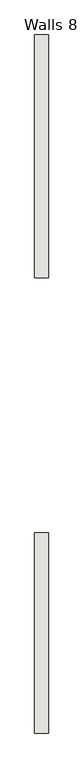
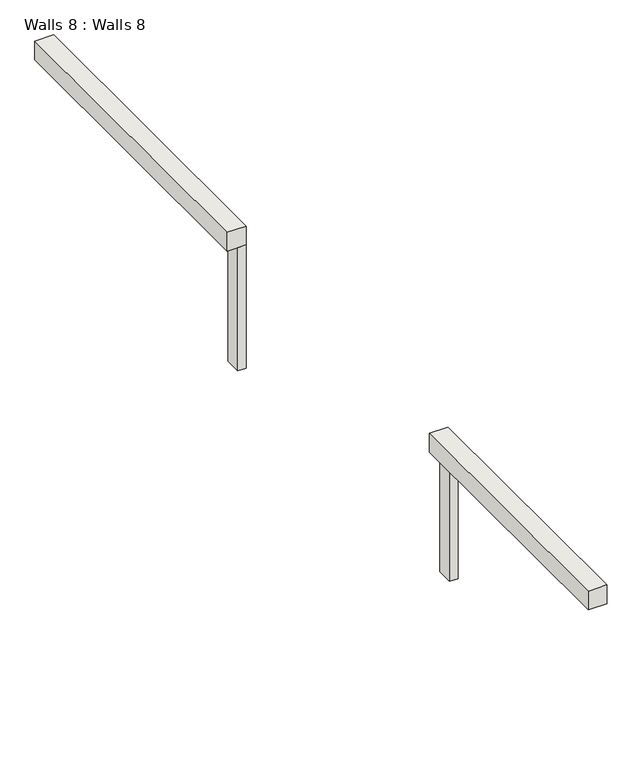
"""IFC4 building model written with IfcOpenShell, lengths in millimetres: wall geometry, Walls 8 : Walls 8."""

from ifc_helpers import new_model, si_unit, frame, origin, place, context, project, spatial, polyline, outline, extrude, source, transform, mapped, element, save


def walls_8_walls_8_d012f144(model_context):
    return source(origin(), model_context, "Body", "SweptSolid", [
        extrude(outline(polyline([(2196.2271302, 3766.5740351), (2196.2271302, 3664.9740351), (2145.4271302, 3664.9740351), (2145.4271302, 3766.5740351), (2196.2271302, 3766.5740351)])), frame((0.0, 0.0, 3962.4), z_axis=(0.0, 0.0, 1.0), x_axis=(1.0, 0.0, 0.0)), (0.0, 0.0, 1.0), 793.75),
        extrude(outline(polyline([(2196.2271302, 6001.7740351), (2196.2271302, 5900.1740351), (2145.4271302, 5900.1740351), (2145.4271302, 6001.7740351), (2196.2271302, 6001.7740351)])), frame((0.0, 0.0, 3962.4), z_axis=(0.0, 0.0, 1.0), x_axis=(1.0, 0.0, 0.0)), (0.0, 0.0, 1.0), 793.75),
        extrude(outline(polyline([(2196.2271302, 3766.5740351), (2196.2271302, 2090.1740351), (2081.9271302, 2090.1740351), (2081.9271302, 3766.5740351), (2196.2271302, 3766.5740351)])), frame((0.0, 0.0, 4756.15), z_axis=(0.0, 0.0, 1.0), x_axis=(1.0, 0.0, 0.0)), (0.0, 0.0, 1.0), 120.65),
        extrude(outline(polyline([(2196.2271302, 7932.1740351), (2196.2271302, 5900.1740351), (2081.9271302, 5900.1740351), (2081.9271302, 7932.1740351), (2196.2271302, 7932.1740351)])), frame((0.0, 0.0, 4756.15), z_axis=(0.0, 0.0, 1.0), x_axis=(1.0, 0.0, 0.0)), (0.0, 0.0, 1.0), 120.65),
    ])


if __name__ == "__main__":
    model = new_model("IFC4")
    model_context = context("Model", 3, world=origin())
    ifc_project = project(units=[si_unit("LENGTHUNIT", "METRE", prefix="MILLI")], contexts=[model_context])
    site = spatial("IfcSite", under=ifc_project)
    building = spatial("IfcBuilding", under=site)
    placement = place(None, origin())
    walls_8_walls_8_shape = walls_8_walls_8_d012f144(model_context)
    element("IfcWall", 1, ObjectType="Walls 8 : Walls 8", at=placement, inside=building, context=model_context, shape_type="MappedRepresentation", body=[
        mapped(walls_8_walls_8_shape, transform((0.0, 0.0, 0.0), x_axis=(1.0, 0.0, 0.0), y_axis=(0.0, 1.0, 0.0), z_axis=(0.0, 0.0, 1.0))),
    ])
    save(model, "model.ifc")

# Revit data of these elements
# Element 1 (IfcWall, "Walls 8 : Walls 8")
#   Materials on its faces: "Default Wall"
# Materials
#   "Default Wall": colour RGB 128 128 128, transparency 0
